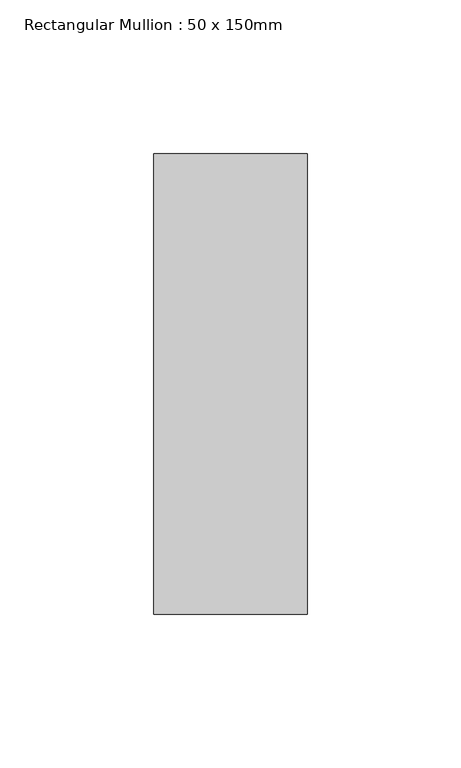
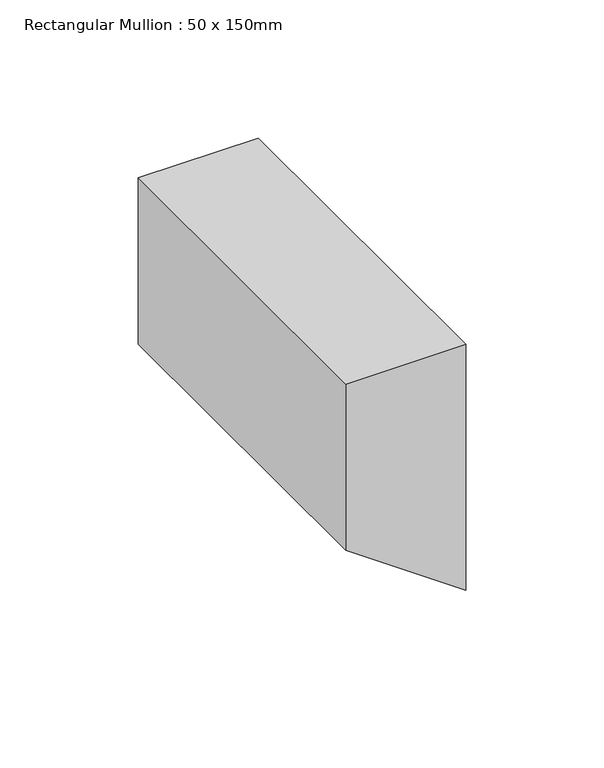
"""IFC4 building model written with IfcOpenShell, lengths in millimetres: member geometry, Rectangular Mullion : 50 x 150mm."""

from ifc_helpers import new_model, si_unit, frame, origin, place, context, project, spatial, polyline, outline, extrude, source, transform, mapped, element, save


def rectangular_mullion_50_x_150mm_e09f09b0(model_context):
    return source(origin(), model_context, "Body", "SweptSolid", [
        extrude(outline(polyline([(0.0, 25.0), (0.0, -25.0), (-73.3380699, -25.0), (-108.3484468, 25.0), (0.0, 25.0)])), frame((0.0, -75.0, 0.0), z_axis=(0.0, 1.0, 0.0), x_axis=(0.0, 0.0, 1.0)), (0.0, 0.0, 1.0), 150.0),
    ])


if __name__ == "__main__":
    model = new_model("IFC4")
    model_context = context("Model", 3, world=origin())
    ifc_project = project(units=[si_unit("LENGTHUNIT", "METRE", prefix="MILLI")], contexts=[model_context])
    site = spatial("IfcSite", under=ifc_project)
    building = spatial("IfcBuilding", under=site)
    placement = place(None, origin())
    rectangular_mullion_50_x_150mm_shape = rectangular_mullion_50_x_150mm_e09f09b0(model_context)
    element("IfcMember", 1, ObjectType="Rectangular Mullion : 50 x 150mm", at=placement, inside=building, context=model_context, shape_type="MappedRepresentation", body=[
        mapped(rectangular_mullion_50_x_150mm_shape, transform((0.0, 0.0, 0.0), x_axis=(1.0, 0.0, 0.0), y_axis=(0.0, 1.0, 0.0), z_axis=(0.0, 0.0, 1.0))),
    ])
    save(model, "model.ifc")

# Revit data of these elements
# Type "Rectangular Mullion : 50 x 150mm"
#   built-in parameter 1007304 = 0.492126 (stored number, unit not read)
#   built-in parameter 1007301 = 0.082021 (stored number, unit not read)
#   built-in parameter 1007300 = 0.082021 (stored number, unit not read)
# Element 1 (IfcMember, "Rectangular Mullion : 50 x 150mm")
#   Materials on its faces: "Aluminium"
# Materials
#   "Aluminium": class "Metal", colour RGB 247 247 247, transparency 0, Description = "Aluminium 6061", Cost = 0
